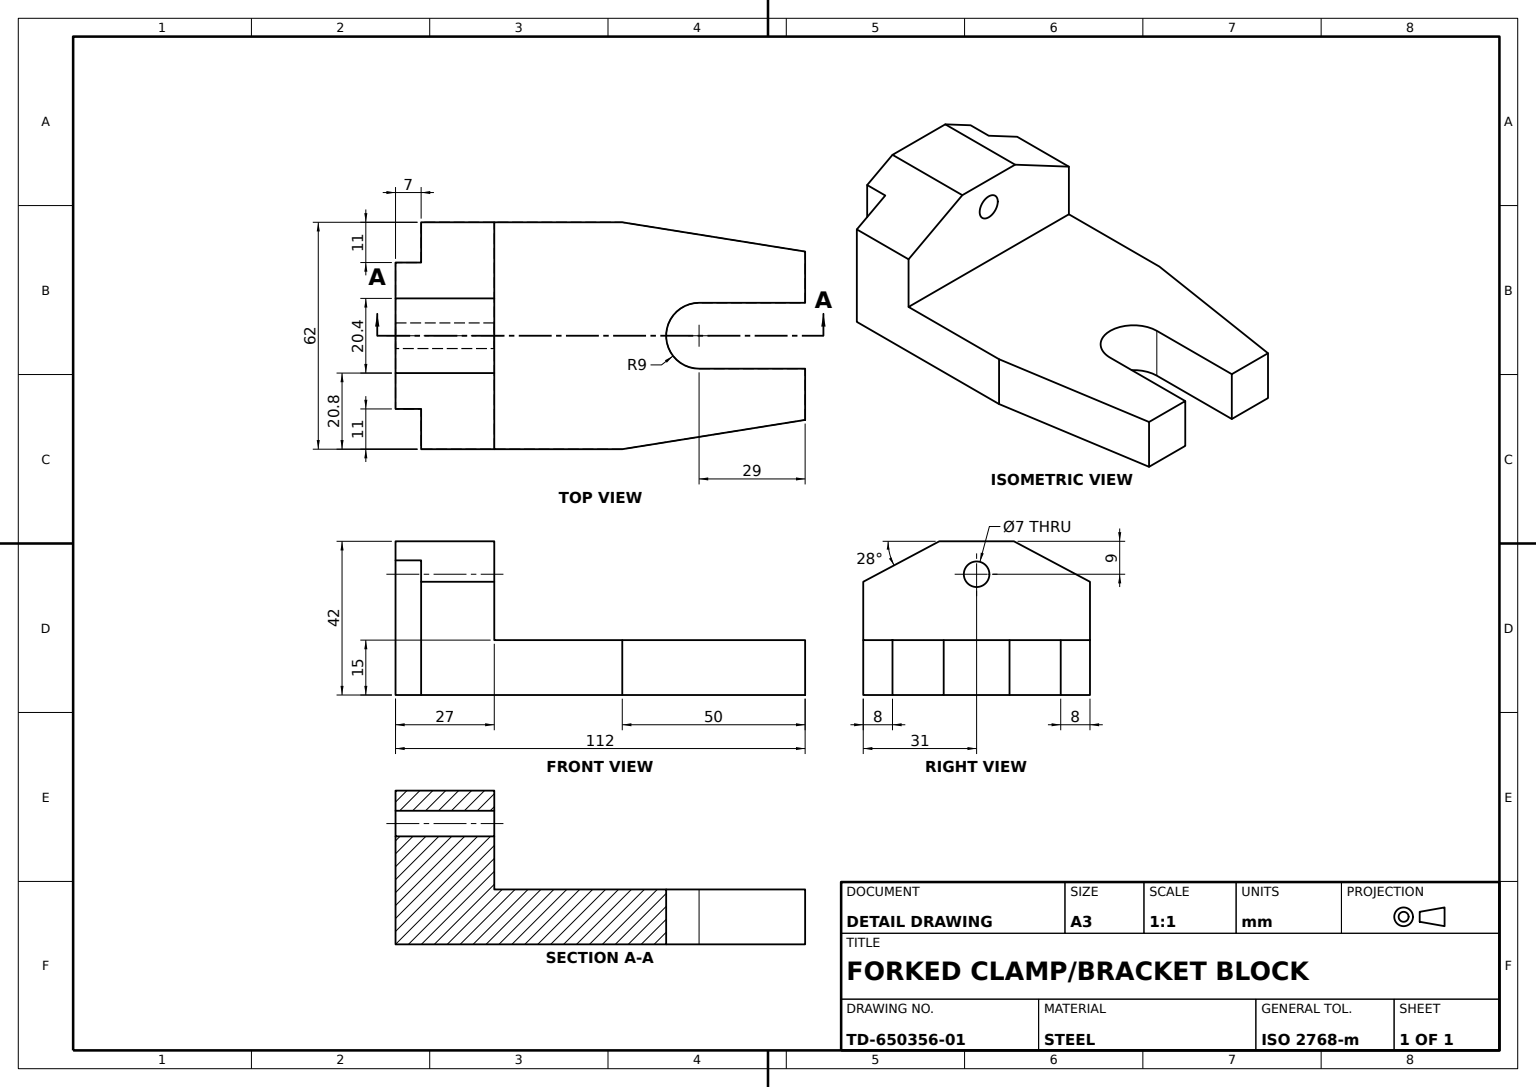
from build123d import *

# Parameters (mm, degrees)
BRACKET_BODY_DEPTH     = 31
HEAD_CHAMFER_SKETCH_R  = 3.5
HEAD_CHAMFER_CUT_DEPTH = 31
HEAD_NOTCH_SKETCH_W    = 7
HEAD_NOTCH_SKETCH_H    = 11
HEAD_NOTCH_CUT_DEPTH   = 51
FORKED_SLOT_CUT_DEPTH  = 102


with BuildPart() as part:
    # Bracket Profile Sketch → Bracket Body (new, symmetric)
    with BuildSketch(Plane.XY):
        Polygon((0, 15), (0, 0), (27, 0), (112, 0), (112, 15), (27, 15), (27, 42), (0, 42), align=None)
    extrude(amount=BRACKET_BODY_DEPTH, both=True)

    # Head Chamfer Sketch → Head Chamfer Cut (cut, symmetric)
    with BuildSketch(Plane(origin=(27, 0, 0), x_dir=(0, 0, -1), z_dir=(1, 0, 0))):
        with Locations(Location((0, 33, 0), (0, 0, 180))):
            Circle(HEAD_CHAMFER_SKETCH_R)
        Polygon((10.202979839, 42), (31, 30.94202823), (31, 54.961145536), (-31, 54.961145536), (-31, 30.940443821), (-10.2, 42), align=None)
    extrude(amount=HEAD_CHAMFER_CUT_DEPTH, both=True, mode=Mode.SUBTRACT)

    # Head Notch Sketch → Head Notch Cut (cut, symmetric)
    with BuildSketch(Plane(origin=(0, 42, 0), x_dir=(1, 0, 0), z_dir=(0, 1, 0))):
        with Locations((3.5, 25.5)):
            Rectangle(HEAD_NOTCH_SKETCH_W, HEAD_NOTCH_SKETCH_H)
        with Locations((3.5, -25.5)):
            Rectangle(HEAD_NOTCH_SKETCH_W, HEAD_NOTCH_SKETCH_H)
    extrude(amount=HEAD_NOTCH_CUT_DEPTH, both=True, mode=Mode.SUBTRACT)

    # Forked Slot Sketch → Forked Slot Cut (cut)
    with BuildSketch(Plane(origin=(0, 15, 0), x_dir=(1, 0, 0), z_dir=(0, 1, 0))):
        Polygon((62, -31), (112, -23), (112, -31), align=None)
        Polygon((62, 31), (112, 23), (112, 31), align=None)
        with BuildLine():
            Line((83, 9), (112, 9))
            Line((112, 9), (112, -9))
            Line((112, -9), (83, -9))
            ThreePointArc((83, -9), (74, 0), (83, 9))
        make_face()
    extrude(amount=-FORKED_SLOT_CUT_DEPTH, mode=Mode.SUBTRACT)


solid = part.part
